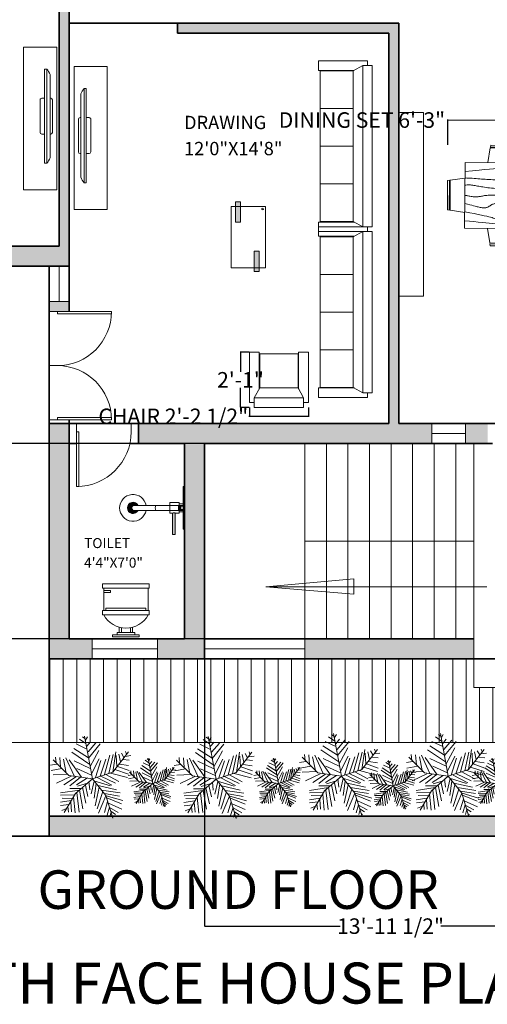
# Model space of a CAD drawing. Units: inches. Extents: x 1319 to 2030, y 219 to 1069.
# Tile 21 of 28: x 1565 to 1776, y 219 to 663. Entities that reach past the tile are written whole.
import ezdxf

# ---------------------------------------------------------------- set-up
doc = ezdxf.new("R2010")
doc.units = ezdxf.units.IN
doc.header["$MEASUREMENT"] = 0
doc.layers.get('0').update_dxf_attribs({"color": 12})
for name, color, linetype, lineweight in [('A-ANNO-DIMS', 2, 'Continuous', 18), ('A-AREA-IDEN', 250, 'Continuous', 18), ('A-FLOR', 8, 'Continuous', 18), ('A-FLOR-CASE', 8, 'Continuous', 18), ('A-FLOR-PATT', 41, 'Continuous', 13), ('A-FLOR-STRS', 7, 'Continuous', 18), ('A-GLAZ', 4, 'Continuous', 18), ('A-WALL-PATT', 252, 'Continuous', 13), ('C-PROP', 7, 'Continuous', 35), ('doors', 252, 'Continuous', 18), ('furniture', 250, 'Continuous', 18), ('lawn', 82, 'Continuous', 13), ('PLUMBING FIXTURES', 252, 'Continuous', 18), ('text', 7, 'Continuous', 25), ('walls', 250, 'Continuous', 35)]:
    doc.layers.add(name, color=color, linetype=linetype, lineweight=lineweight)
doc.styles.get("Standard").update_dxf_attribs({"font": 'arial.ttf'})
doc.dimstyles.get("Standard").update_dxf_attribs({"dimtxt": 7, "dimasz": 0.18, "dimexe": 0.18, "dimexo": 0.0625, "dimgap": 0.09, "dimtad": 0, "dimtih": 1, "dimtoh": 1, "dimzin": 0, "dimdsep": 46, "dimlunit": 3, "dimtxsty": 'Standard', "dimcen": 0.09, "dimadec": 0, "dimazin": 0, "dimtfac": 1, "dimtofl": 0, "dimtmove": 0, "dimatfit": 3, "dimfxl": 1, "dimtolj": 1, "dimtzin": 0, "dimarcsym": 0})

# ---------------------------------------------------------------- blocks, each defined once
blk = doc.blocks.new('*U2')
for p, q in [((0, 0), (0, -6)), ((40, 0), (40, -6))]:
    blk.add_line(p, q)
blk.add_lwpolyline([(0, 0), (0, 40), (1.75, 40), (1.75, 0)], close=True)
blk.add_arc((0, 0), 40, 0, 90)
blk = doc.blocks.new('Dining Set - 36 x 72 in.')
for p, q in [((-22, 27.5), (-22.1562, 26.50042)), ((-22, 27.5), (-6, 27.5)), ((-5.8437, 26.49966), (-6, 27.5)), ((6, 27.5), (5.8438, 26.50042)), ((6, 27.5), (22, 27.5)), ((22.1563, 26.49966), (22, 27.5)), ((-22.2343, 26.00059), (-23.4847, 17.99762)), ((-22.2304, 26), (-5.7608, 26)), ((-5.8416, 26.5), (-22.1534, 26.5)), ((-4.5152, 17.99762), (-5.7655, 25.99926)), ((5.7657, 26.00059), (4.5153, 17.99762)), ((5.7696, 26), (22.2392, 26)), ((22.1584, 26.5), (5.8466, 26.5)), ((23.4848, 17.99762), (22.2345, 25.99926)), ((36, 18), (-36, 18)), ((-36, 18), (-36, -18)), ((36, -18), (36, 18)), ((-45.5, 8), (-44.5004, 8.15617)), ((-45.5, 8), (-45.5, -8)), ((-44.5, -8.15843), (-44.5, 8.15338)), ((-44.0006, 8.23428), (-35.9976, 9.48474)), ((-44, 8.23041), (-44, -8.23915)), ((44.0006, 8.23428), (35.9976, 9.48474)), ((44, 8.23041), (44, -8.23915)), ((44.5, -8.15843), (44.5, 8.15338)), ((45.5, 8), (44.5005, 8.15617)), ((45.5, 8), (45.5, -8)), ((-44.4997, -8.15631), (-45.5, -8)), ((-35.9976, -9.48476), (-43.9993, -8.2345)), ((35.9976, -9.48476), (43.9993, -8.2345)), ((44.4997, -8.15631), (45.5, -8)), ((-36, -18), (36, -18)), ((-22.2343, -26.0006), (-23.4847, -17.99762)), ((-4.5152, -17.99762), (-5.7655, -25.99928)), ((5.7657, -26.0006), (4.5153, -17.99762)), ((23.4848, -17.99762), (22.2345, -25.99928)), ((-22.2304, -26), (-5.7608, -26)), ((-22, -27.5), (-22.1562, -26.50044)), ((-5.8416, -26.5), (-22.1534, -26.5)), ((-5.8437, -26.49967), (-6, -27.5)), ((5.7696, -26), (22.2392, -26)), ((6, -27.5), (5.8438, -26.50044)), ((22.1584, -26.5), (5.8466, -26.5)), ((22.1563, -26.49967), (22, -27.5)), ((-22, -27.5), (-6, -27.5)), ((6, -27.5), (22, -27.5))]:
    blk.add_line(p, q)
for points in [[(-36, 15), (-31.1772, 14.97754), (-26.8079, 14.91406), (-22.8538, 14.81543), (-19.276, 14.6875), (-16.0362, 14.53613), (-13.0957, 14.36718), (-10.4159, 14.18652), (-7.9583, 14), (-5.6904, 13.81315), (-3.6035, 13.63021), (-1.6954, 13.45508), (0.0365, 13.29166), (1.5945, 13.14388), (2.9811, 13.01562), (4.1988, 12.9108), (5.25, 12.83333), (6.1393, 12.78613), (6.8802, 12.76823), (7.4883, 12.77767), (7.9792, 12.8125), (8.3685, 12.87077), (8.6719, 12.95052), (8.9049, 13.0498), (9.0833, 13.16666), (9.2205, 13.29899), (9.3216, 13.44401), (9.3895, 13.59879), (9.4271, 13.76041), (9.4373, 13.92594), (9.4232, 14.09245), (9.3875, 14.257), (9.3333, 14.41666), (9.2638, 14.56917), (9.1836, 14.71484), (9.0975, 14.85465), (9.0104, 14.98958), (8.9272, 15.1206), (8.8529, 15.2487), (8.7922, 15.37483), (8.75, 15.5), (8.7305, 15.62467), (8.7344, 15.74739), (8.7617, 15.86621), (8.8125, 15.97916), (8.8867, 16.08431), (8.9844, 16.17968), (9.1055, 16.26334), (9.25, 16.33333), (9.4189, 16.38802), (9.6172, 16.42708), (9.8506, 16.45052), (10.125, 16.45833), (10.4463, 16.45052), (10.8203, 16.42708), (11.2529, 16.38802), (11.75, 16.33333), (12.3184, 16.26318), (12.9694, 16.17838), (13.7151, 16.07991), (14.5677, 15.96875), (15.5395, 15.84586), (16.6426, 15.71224), (17.8893, 15.56884), (19.2917, 15.41666), (20.859, 15.25667), (22.5879, 15.08984), (24.4721, 14.91715), (26.5052, 14.73958), (28.6809, 14.5581), (30.9929, 14.3737), (33.4347, 14.18733), (36, 14)], [(-36, 10), (-28.9766, 10.14274), (-23.1725, 10.20442), (-18.4241, 10.19775), (-14.5677, 10.13541), (-11.4399, 10.03011), (-8.877, 9.89453), (-6.7154, 9.74137), (-4.7917, 9.58333), (-2.9698, 9.43082), (-1.2246, 9.28515), (0.4415, 9.14534), (2.026, 9.01041), (3.5266, 8.87939), (4.9408, 8.7513), (6.266, 8.62516), (7.5, 8.5), (8.6411, 8.37549), (9.6914, 8.2539), (10.6538, 8.13818), (11.5312, 8.03125), (12.3267, 7.93603), (13.043, 7.85547), (13.6831, 7.79248), (14.25, 7.75), (14.7471, 7.7303), (15.1797, 7.73307), (15.5537, 7.75732), (15.875, 7.80208), (16.1494, 7.86637), (16.3828, 7.94922), (16.5811, 8.04964), (16.75, 8.16666), (16.8944, 8.29915), (17.0143, 8.44531), (17.1089, 8.60319), (17.1771, 8.77083), (17.218, 8.94629), (17.2305, 9.1276), (17.2137, 9.31282), (17.1667, 9.5), (17.0895, 9.6875), (16.987, 9.875), (16.8649, 10.0625), (16.7292, 10.25), (16.5856, 10.4375), (16.4401, 10.625), (16.2985, 10.8125), (16.1667, 11), (16.05, 11.18733), (15.9518, 11.3737), (15.8752, 11.5581), (15.8229, 11.73958), (15.798, 11.91715), (15.8034, 12.08984), (15.842, 12.25667), (15.9167, 12.41666), (16.0295, 12.56836), (16.1784, 12.70833), (16.3605, 12.83268), (16.5729, 12.9375), (16.8127, 13.01888), (17.0768, 13.07291), (17.3625, 13.0957), (17.6667, 13.08333), (17.9894, 13.03312), (18.3418, 12.94726), (18.7382, 12.82918), (19.1927, 12.68229), (19.7195, 12.51001), (20.3327, 12.31575), (21.0465, 12.10294), (21.875, 11.875), (22.8357, 11.63354), (23.959, 11.37304), (25.2786, 11.08618), (26.8282, 10.76562), (28.6414, 10.40405), (30.752, 9.99414), (33.1936, 9.52856), (36, 9)], [(-36, 5.5), (-30.7157, 5.3348), (-26.069, 5.20963), (-21.9946, 5.11767), (-18.4271, 5.05208), (-15.3009, 5.00602), (-12.5508, 4.97265), (-10.1112, 4.94515), (-7.9167, 4.91666), (-5.909, 4.88167), (-4.0586, 4.83984), (-2.3429, 4.79215), (-0.7396, 4.73958), (0.7739, 4.6831), (2.22, 4.6237), (3.6213, 4.56233), (5, 4.5), (6.373, 4.43782), (7.7344, 4.3776), (9.0723, 4.32129), (10.375, 4.27083), (11.6309, 4.22819), (12.8281, 4.19531), (13.9551, 4.17415), (15, 4.16666), (15.954, 4.17448), (16.819, 4.19791), (17.6001, 4.23698), (18.3021, 4.29166), (18.9299, 4.36198), (19.4883, 4.44791), (19.9823, 4.54948), (20.4167, 4.66666), (20.7969, 4.79899), (21.1302, 4.94401), (21.4245, 5.09879), (21.6875, 5.26041), (21.9271, 5.42594), (22.1511, 5.59245), (22.3672, 5.757), (22.5834, 5.91666), (22.8065, 6.06868), (23.0404, 6.21093), (23.2879, 6.34147), (23.5521, 6.45833), (23.8358, 6.55957), (24.142, 6.64323), (24.4735, 6.70735), (24.8334, 6.75), (25.2235, 6.76969), (25.642, 6.76692), (26.0858, 6.74267), (26.5521, 6.69791), (27.0379, 6.63362), (27.5404, 6.55078), (28.0565, 6.45036), (28.5834, 6.33333), (29.1242, 6.19987), (29.7071, 6.04687), (30.3661, 5.87044), (31.1354, 5.66666), (32.0493, 5.43164), (33.142, 5.16146), (34.4475, 4.85221), (36, 4.5)], [(-36, -1), (-30.7915, -0.6591), (-26.0195, -0.38216), (-21.6519, -0.16284), (-17.6563, 0.00521), (-14.0005, 0.12833), (-10.6523, 0.21289), (-7.5796, 0.26522), (-4.75, 0.29166), (-2.134, 0.29793), (0.2878, 0.28711), (2.5317, 0.26163), (4.6146, 0.22396), (6.5529, 0.17651), (8.3633, 0.12174), (10.0623, 0.06209), (11.6667, 0), (13.1899, -0.06201), (14.6341, -0.1211), (15.9982, -0.17432), (17.2813, -0.21875), (18.4823, -0.25147), (19.6003, -0.26953), (20.6343, -0.27002), (21.5834, -0.25), (22.4481, -0.20768), (23.2357, -0.14584), (23.9549, -0.06836), (24.6146, 0.02083), (25.2235, 0.11784), (25.7904, 0.21875), (26.3241, 0.31966), (26.8334, 0.41666), (27.3265, 0.50618), (27.8099, 0.58593), (28.2894, 0.65397), (28.7709, 0.70833), (29.2601, 0.74707), (29.763, 0.76823), (30.2855, 0.76985), (30.8334, 0.75), (31.4088, 0.70784), (31.9994, 0.64713), (32.589, 0.57275), (33.1615, 0.48958), (33.7008, 0.4025), (34.1908, 0.3164), (34.6153, 0.23616), (34.9584, 0.16666), (35.2099, 0.11165), (35.3848, 0.07031), (35.504, 0.04069), (35.5886, 0.02083), (35.6594, 0.00879), (35.7377, 0.0026), (35.8442, 0.00032), (36, 0)], [(-36, -6.5), (-27.1843, -6.31267), (-20.084, -6.1263), (-14.469, -5.9419), (-10.1094, -5.76042), (-6.7752, -5.58285), (-4.2363, -5.41016), (-2.2629, -5.24333), (-0.625, -5.08334), (0.8708, -4.93099), (2.2715, -4.78646), (3.5872, -4.64974), (4.8281, -4.52084), (6.0046, -4.39974), (7.127, -4.28646), (8.2053, -4.18099), (9.25, -4.08334), (10.2705, -3.99382), (11.2734, -3.91407), (12.2647, -3.84603), (13.25, -3.79167), (14.2354, -3.75293), (15.2266, -3.73177), (16.2295, -3.73015), (17.25, -3.75), (18.2912, -3.79248), (19.3451, -3.85547), (20.4009, -3.93604), (21.4479, -4.03125), (22.4754, -4.13819), (23.4727, -4.25391), (24.4289, -4.37549), (25.3334, -4.5), (26.1785, -4.62492), (26.9694, -4.74935), (27.7145, -4.87281), (28.4219, -4.99479), (29.1, -5.11483), (29.7572, -5.23242), (30.4016, -5.34709), (31.0417, -5.45834), (31.6837, -5.56437), (32.3262, -5.65821), (32.9658, -5.73153), (33.599, -5.77604), (34.2224, -5.78345), (34.8327, -5.74545), (35.4264, -5.65373), (36, -5.5)], [(-36, -10), (-26.4022, -9.81299), (-18.4675, -9.62891), (-11.9839, -9.45069), (-6.7396, -9.28125), (-2.5226, -9.12354), (0.8789, -8.98047), (3.6769, -8.85498), (6.0833, -8.75), (8.2767, -8.66765), (10.3021, -8.60677), (12.1712, -8.56543), (13.8958, -8.54167), (15.4876, -8.53353), (16.9583, -8.53907), (18.3197, -8.55632), (19.5834, -8.58334), (20.7616, -8.61841), (21.8685, -8.66081), (22.9188, -8.71004), (23.9271, -8.76563), (24.9081, -8.82707), (25.8763, -8.89388), (26.8465, -8.96558), (27.8334, -9.04167), (28.8474, -9.12118), (29.8828, -9.20117), (30.93, -9.27824), (31.9792, -9.34896), (33.0205, -9.40991), (34.0443, -9.45768), (35.0407, -9.48885), (36, -9.5)], [(-36, -14.5), (-30.0881, -14.33513), (-25.0332, -14.21224), (-20.7312, -14.12647), (-17.0781, -14.07292), (-13.97, -14.04671), (-11.3027, -14.04297), (-8.9724, -14.05681), (-6.875, -14.08334), (-4.9224, -14.11833), (-3.0905, -14.16016), (-1.3709, -14.20785), (0.2448, -14.26042), (1.7647, -14.3169), (3.1973, -14.3763), (4.5507, -14.43767), (5.8333, -14.5), (7.0554, -14.5621), (8.235, -14.62175), (9.3922, -14.67652), (10.5469, -14.72396), (11.7192, -14.76164), (12.929, -14.78711), (14.1965, -14.79794), (15.5417, -14.79167), (16.9933, -14.76424), (18.6152, -14.70508), (20.4804, -14.60197), (22.6615, -14.44271), (25.2312, -14.21509), (28.2624, -13.9069), (31.8277, -13.50594), (36, -13)]]:
    blk.add_lwpolyline(points)
blk = doc.blocks.new('dining area')
at = {"layer": 'furniture', "xscale": 0.6659924291999282, "yscale": 0.6659924291999282, "zscale": 0.6659924291999282, "rotation": 90}
blk.add_blockref('Dining Set - 36 x 72 in.', (-0.44, 20.51), dxfattribs=at)
blk = doc.blocks.new('FABRIC SOFA 1S')
at = {"layer": 'furniture'}
for p, q in [((0, -15.12), (0, 15.12)), ((6, 15.12), (0, 15.12)), ((3, 18.12), (34, 18.12)), ((3, 15.12), (3, 18.12)), ((6, -15.12), (6, 15.12)), ((12, 11.75), (6, 15.12)), ((11.33, 12.12), (34, 12.12)), ((34, 12.12), (34, 18.12)), ((6, -15.12), (12, -11.75)), ((6, -15.12), (0, -15.12)), ((3, -18.12), (3, -15.12)), ((3, -18.12), (34, -18.12)), ((11.33, -12.12), (34, -12.12)), ((34, -12.12), (34, -18.12))]:
    blk.add_line(p, q, dxfattribs=at)
blk.add_lwpolyline([(12, -11.75), (12, 11.75), (33, 11.75), (33, -11.75)], close=True, dxfattribs=at)
blk = doc.blocks.new('FABRIC SOFA 4S')
at = {"layer": 'furniture'}
for p, q in [((0, -51), (0, 51)), ((6, 51), (0, 51)), ((3, 54), (34, 54)), ((3, 51), (3, 54)), ((6, -51), (6, 51)), ((12, 47.63), (6, 51)), ((34, 48), (34, 54)), ((11.14, 48), (34, 48)), ((33, 23.81), (12, 23.81)), ((33, 0), (12, 0)), ((33, -23.81), (12, -23.81)), ((6, -51), (12, -47.63)), ((11.54, -48), (34, -48)), ((34, -48), (34, -54)), ((6, -51), (0, -51)), ((3, -54), (3, -51)), ((3, -54), (34, -54))]:
    blk.add_line(p, q, dxfattribs=at)
blk.add_lwpolyline([(12, -47.63), (12, 47.63), (33, 47.63), (33, -47.63)], close=True, dxfattribs=at)
blk = doc.blocks.new('O.H SHOWER-PL')
at = {"layer": 'PLUMBING FIXTURES'}
for points in [[(-1.84, 0), (-1.84, -0.25), (1.84, -0.25), (1.84, 0)], [(0.46, -8.72), (0.46, -9.67, -0.422337), (-0.46, -9.67), (-0.46, -8.72, 4.325472)]]:
    blk.add_hatch(color=256, dxfattribs=at).paths.add_polyline_path(points)
for p, q in [((-1.84, 0), (-1.84, -0.25)), ((1.84, 0), (-1.84, 0)), ((1.84, 0), (1.84, -0.25)), ((1.84, -0.25), (-1.84, -0.25)), ((-0.46, -0.25), (-0.46, -9.67)), ((0.46, -0.25), (0.46, -9.67))]:
    blk.add_line(p, q, dxfattribs=at)
for centre, radius, start, end in [((0, -4.48), 1.03, 243.53, 296.47), ((0, -9.67), 2.5, 100.61, 79.39), ((0, -9.67), 1.05, 116.0349, 63.9652), ((0, -9.22), 0.643, 224.2078, 315.7922)]:
    blk.add_arc(centre, radius, start, end, dxfattribs=at)
blk = doc.blocks.new('DIVERTER-PL')
at = {"layer": 'PLUMBING FIXTURES'}
for points in [[(4, 0), (-4, 0), (-4, -0.25), (4, -0.25)], [(0.38, -1.14), (0.38, -0.7), (-0.37, -0.7), (-0.37, -1.14)], [(1, -1.75, 0.30818), (1, -2.25), (5, -2.25), (5, -1.75)]]:
    blk.add_hatch(color=256, dxfattribs=at).paths.add_polyline_path(points)
for p, q in [((-4, 0), (-4, -0.25)), ((-4, 0), (4, 0)), ((4, 0), (4, -0.25)), ((-4, -0.25), (4, -0.25)), ((-4, -0.25), (4, -0.25)), ((-1, -1.05), (-0.37, -1.05)), ((-1, -1.05), (-1, -2.75)), ((-0.75, -0.25), (-0.75, -1.05)), ((-0.37, -0.7), (0.38, -0.7)), ((-0.37, -0.7), (-0.37, -1.14)), ((-0.37, -1.14), (0.38, -1.14)), ((-0.32, -0.7), (-0.32, -0.25)), ((0.32, -0.7), (0.32, -0.25)), ((0.38, -0.7), (0.38, -1.14)), ((0.38, -1.05), (1, -1.05)), ((0.75, -0.25), (0.75, -1.05)), ((1, -1.05), (1, -1.75)), ((-1, -2.75), (1, -2.75)), ((1, -2.25), (1, -2.75))]:
    blk.add_line(p, q, dxfattribs=at)
at = {"layer": 'PLUMBING FIXTURES', "ltscale": 12}
for p, q in [((1, -1.75), (5, -1.75)), ((5, -2.25), (5, -1.75)), ((1, -2.25), (5, -2.25))]:
    blk.add_line(p, q, dxfattribs=at)
at = {"layer": 'PLUMBING FIXTURES'}
blk.add_arc((1.37, -2), 0.444, 145.7435, 214.2565, dxfattribs=at)
blk = doc.blocks.new('A$C7F153053')
at = {"layer": 'PLUMBING FIXTURES', "xscale": -1, "rotation": 270}
for name in ['DIVERTER-PL', 'O.H SHOWER-PL']:
    blk.add_blockref(name, (12.17, 4), dxfattribs=at)
blk = doc.blocks.new('*U25')
for p, q in [((-10, 22), (-10, 12)), ((-10, 21), (-7, 21)), ((-7, 20), (-10, 20)), ((-7, 21), (-7, 20)), ((10, 12), (10, 22)), ((10.5, 12), (-10.5, 12)), ((-10.5, 10), (-10.5, 12)), ((10.5, 10), (-10.5, 10)), ((9, 13), (-9, 13)), ((-9, 13), (-9, 12)), ((9, 12), (9, 13)), ((10.5, 12), (10.5, 10)), ((4, 2), (-4, 2)), ((-4, 2), (-4, 1)), ((-3, 4.4065), (-3, 2)), ((-2, 2), (-2, 4.1658)), ((2, 4.1658), (2, 2)), ((3, 2), (3, 4.4065)), ((4, 1), (4, 2))]:
    blk.add_line(p, q)
for points in [[(10.5, 22), (10.5, 24), (-10.5, 24), (-10.5, 22)], [(6, 0), (6, 1), (-6, 1), (-6, 0)]]:
    blk.add_lwpolyline(points, close=True)
blk.add_arc((0, 15.3333), 11.3333, 208.0725, 331.9275)
blk = doc.blocks.new('*U27')
for p, q in [((-8.737, 47.138), (-17.069, 52.711)), ((-10.186, 53.64), (-13.084, 55.962)), ((0, 0), (-10.5, 57)), ((-9.099, 51.782), (-6.563, 55.962)), ((-5.114, 28.097), (-24.676, 40.636)), ((-7.288, 39.707), (-21.778, 46.673)), ((-7.65, 43.423), (-2.578, 49.46)), ((-5.839, 35.992), (4.667, 48.067)), ((-5.114, 27.632), (10.463, 46.673)), ((-48.585, 21.131), (-49.309, 29.026)), ((-43.513, 28.561), (-42.427, 15.558)), ((-35.544, 28.097), (-24.314, 3.947)), ((-3.665, 19.273), (-27.574, 35.527)), ((-2.941, 16.486), (8.652, 37.85)), ((-1.129, 6.734), (9.014, 26.704)), ((16.259, 5.805), (23.142, 31.348)), ((22.055, 7.198), (27.489, 32.277)), ((27, 9), (48, 36)), ((27.127, 9.056), (31.112, 35.992)), ((31.836, 30.883), (32.561, 16.486)), ((35.096, 32.741), (37.27, 22.524)), ((38.719, 34.134), (41.979, 28.561)), ((43.791, 29.954), (51.036, 30.883)), ((44.153, 36.456), (45.239, 32.741)), ((-47.498, 19.737), (-55.83, 18.344)), ((-40.615, 13.7), (-55.105, 10.913)), ((-31.5, 4.5), (-52.5, 25.5)), ((-38.442, 26.239), (-34.819, 7.663)), ((-14.533, 2.09), (-30.834, 25.31)), ((-24.314, 23.917), (-2.941, 13.7)), ((-20.691, 13.7), (-1.129, 4.876)), ((3.942, 1.625), (11.187, 24.381)), ((10.101, 3.483), (17.708, 26.239)), ((33.285, 16.486), (48.862, 10.913)), ((36.183, 19.737), (48.137, 17.88)), ((40.53, 25.775), (48.862, 24.846)), ((-33.37, 6.269), (-52.207, 5.34)), ((-28.299, 3.483), (-47.86, -5.805)), ((-21.416, 3.018), (-38.079, -8.128)), ((0, 0), (-31.5, 4.5)), ((-15.982, 2.09), (-30.11, -9.521)), ((0, 0), (-22.5, -19.5)), ((-6.563, 1.161), (-21.416, -8.128)), ((0, 0), (27, 9)), ((0, 0), (18, -22.5)), ((6.478, 1.625), (26.04, -8.592)), ((11.187, 3.483), (30.749, -5.805)), ((18.07, 5.805), (35.096, -3.483)), ((24.229, 7.663), (46.688, 1.625)), ((29.662, 12.307), (48.137, 6.269)), ((-15.257, -12.772), (-30.11, -12.772)), ((-6.563, -5.805), (-19.967, -9.985)), ((-13.446, -11.378), (-8.737, -32.741)), ((-9.461, -8.592), (-6.201, -23.453)), ((-4.752, -3.483), (-3.665, -14.629)), ((2.493, -3.019), (-1.491, -20.202)), ((1.769, -2.555), (24.229, -9.521)), ((5.029, -6.27), (2.131, -25.775)), ((9.014, -11.378), (3.58, -35.992)), ((7.565, -9.056), (32.198, -14.629)), ((-17.431, -15.094), (-42.789, -18.809)), ((-24.314, -21.596), (-42.427, -22.06)), ((-26.849, -26.24), (-40.253, -25.775)), ((-22.5, -19.5), (-37.5, -45)), ((-25.038, -23.918), (-22.865, -45.281)), ((-20.691, -18.345), (-17.793, -44.352)), ((-17.069, -15.094), (-12.721, -40.172)), ((14.085, -16.951), (6.478, -40.172)), ((18.07, -22.524), (8.289, -45.745)), ((12.274, -15.094), (36.907, -18.809)), ((16.259, -19.738), (36.183, -22.989)), ((18, -22.5), (27, -52.5)), ((18.433, -22.524), (40.53, -29.026)), ((19.157, -25.311), (38.719, -33.206)), ((-28.299, -29.026), (-42.789, -31.348)), ((-30.834, -34.135), (-42.427, -35.528)), ((-32.646, -36.921), (-31.921, -44.352)), ((-29.023, -30.884), (-27.936, -43.887)), ((20.244, -30.419), (15.897, -44.816)), ((22.78, -37.85), (19.519, -48.532)), ((21.331, -32.741), (39.081, -40.636)), ((22.78, -38.314), (34.372, -44.816)), ((-34.457, -39.708), (-40.978, -42.494)), ((24.591, -45.745), (23.142, -50.854)), ((24.591, -43.423), (30.749, -47.603)), ((26.764, -49.925), (28.213, -50.854))]:
    blk.add_line(p, q)
blk = doc.blocks.new('TABLE-COCKTAIL')
h = blk.add_hatch(color=256)
h.dxf.hatch_style = 1
h.paths.add_polyline_path([(4.23, 29.31), (2.04, 29.31), (2.04, 22.19), (4.23, 22.19)])
h.paths.add_polyline_path([(4.23, 31.28), (2.04, 31.28), (2.04, 29.31), (4.23, 29.31)])
h.paths.add_polyline_path([(12.58, 9.09), (10.39, 9.09), (10.39, 1.62), (12.58, 1.62)])
h.paths.add_polyline_path([(12.58, 1.62), (10.39, 1.62), (10.39, 0), (12.58, 0)])
for p, q in [((2.04, 31.28), (4.23, 31.28)), ((2.04, 22.19), (2.04, 31.28)), ((4.23, 31.28), (4.23, 22.19)), ((0, 29.31), (0, 1.62)), ((15.53, 29.31), (0, 29.31)), ((15.53, 1.62), (15.53, 29.31)), ((4.23, 22.19), (2.04, 22.19)), ((10.39, 9.09), (12.58, 9.09)), ((10.39, 0), (10.39, 9.09)), ((12.58, 9.09), (12.58, 0)), ((0, 1.62), (15.53, 1.62)), ((12.58, 0), (10.39, 0))]:
    blk.add_line(p, q)
blk.add_circle((14.17, 28.1), 0.401)
blk = doc.blocks.new('PLASMA-LARGE')
at = {"layer": 'furniture'}
for p, q in [((-7.26, 0), (7.26, 0)), ((-21, -2.5), (21, -2.5)), ((-21, -2.5), (-21, -3.5)), ((-21, -3.5), (21, -3.5)), ((-18.61, -1), (18.61, -1)), ((-8, -1), (-8, -0.74)), ((-8, -3.5), (-8, -4.76)), ((8, -1), (8, -0.74)), ((8, -3.5), (8, -4.76)), ((21, -2.5), (21, -3.5)), ((-7.26, -5.5), (7.26, -5.5))]:
    blk.add_line(p, q, dxfattribs=at)
for centre, radius, start, end in [((-7.26, -0.74), 0.744, 90, 180), ((7.26, -0.74), 0.744, 0, 90), ((-13.97, -11.05), 11.07, 114.7602, 129.4175), ((13.97, -11.05), 11.07, 50.5825, 65.2398), ((-7.26, -4.76), 0.744, 180, 270), ((7.26, -4.76), 0.744, 270, 0)]:
    blk.add_arc(centre, radius, start, end, dxfattribs=at)
blk = doc.blocks.new('MEDIA-CONSOLE')
for p, q in [((64.44, 14.9), (0, 14.9)), ((0, 14.9), (0, 0)), ((64.44, 0), (64.44, 14.9)), ((0, 0), (64.44, 0))]:
    blk.add_line(p, q)
at = {"xscale": -1.011294184530666, "yscale": 1.011294184530666, "zscale": 1.011294184530666, "rotation": 180}
blk.add_blockref('PLASMA-LARGE', (33.26, 1.95), dxfattribs=at)
blk = doc.blocks.new('*D54')
at = {"layer": 'A-ANNO-DIMS', "color": 0, "lineweight": -2, "transparency": 16777216}
for p, q in [((1757.94, 618.08), (1757.76, 618.08)), ((1757.87, 606.9), (1757.94, 618.26)), ((1832.71, 617.63), (1758.12, 618.08)), ((1832.82, 606.45), (1832.89, 617.81))]:
    blk.add_line(p, q, dxfattribs=at)
at = {"layer": 'A-ANNO-DIMS', "color": 0, "transparency": 16777216}
for points in [[(1758.12, 618.11), (1758.12, 618.05), (1757.94, 618.08)], [(1832.71, 617.66), (1832.71, 617.6), (1832.89, 617.63)]]:
    blk.add_solid(points, dxfattribs=at)
at = {"layer": 'Defpoints', "color": 0, "transparency": 16777216}
for p in [(1757.94, 618.08), (1757.87, 606.84), (1832.82, 606.38)]:
    blk.add_point(p, dxfattribs=at)
at = {"layer": 'A-ANNO-DIMS', "color": 0, "transparency": 16777216, "insert": (1719.2, 618.08), "char_height": 7, "attachment_point": 5}
blk.add_mtext('\\A1;DINING SET 6\'-3"', dxfattribs=at)
blk = doc.blocks.new('*D60')
at = {"layer": 'A-ANNO-DIMS', "color": 0, "lineweight": -2, "transparency": 16777216}
for p, q in [((1668.5, 488.43), (1668.5, 484.32)), ((1695.11, 488.43), (1695.11, 484.32)), ((1668.5, 484.5), (1668.32, 484.5)), ((1694.93, 484.5), (1668.68, 484.5))]:
    blk.add_line(p, q, dxfattribs=at)
at = {"layer": 'A-ANNO-DIMS', "color": 0, "transparency": 16777216}
for points in [[(1668.68, 484.53), (1668.68, 484.47), (1668.5, 484.5)], [(1694.93, 484.53), (1694.93, 484.47), (1695.11, 484.5)]]:
    blk.add_solid(points, dxfattribs=at)
at = {"layer": 'Defpoints', "color": 0, "transparency": 16777216}
for p in [(1668.5, 488.49), (1695.11, 488.49), (1668.5, 484.5)]:
    blk.add_point(p, dxfattribs=at)
at = {"layer": 'A-ANNO-DIMS', "color": 0, "transparency": 16777216, "insert": (1634.24, 484.5), "char_height": 7, "attachment_point": 5}
blk.add_mtext('\\A1;CHAIR 2\'-2 1/2"', dxfattribs=at)
blk = doc.blocks.new('*D61')
at = {"layer": 'A-ANNO-DIMS', "color": 0, "lineweight": -2, "transparency": 16777216}
for p, q in [((1668.44, 513.45), (1664.33, 513.45)), ((1664.51, 513.27), (1664.51, 504.58)), ((1664.51, 488.67), (1664.51, 497.37)), ((1668.44, 488.49), (1664.33, 488.49))]:
    blk.add_line(p, q, dxfattribs=at)
at = {"layer": 'A-ANNO-DIMS', "color": 0, "transparency": 16777216}
for points in [[(1664.48, 513.27), (1664.54, 513.27), (1664.51, 513.45)], [(1664.48, 488.67), (1664.54, 488.67), (1664.51, 488.49)]]:
    blk.add_solid(points, dxfattribs=at)
at = {"layer": 'Defpoints', "color": 0, "transparency": 16777216}
for p in [(1664.51, 513.45), (1668.5, 513.45), (1668.5, 488.49)]:
    blk.add_point(p, dxfattribs=at)
at = {"layer": 'A-ANNO-DIMS', "color": 0, "transparency": 16777216, "insert": (1664.51, 500.97), "char_height": 7, "attachment_point": 5}
blk.add_mtext('\\A1;2\'-1"', dxfattribs=at)
blk = doc.blocks.new('*D64')
at = {"layer": 'A-ANNO-DIMS', "color": 0, "lineweight": -2, "transparency": 16777216}
for p, q in [((1648.34, 375.16), (1648.34, 254.5)), ((1815.84, 375.16), (1815.84, 254.5)), ((1648.52, 254.68), (1709.43, 254.68)), ((1815.66, 254.68), (1754.75, 254.68))]:
    blk.add_line(p, q, dxfattribs=at)
at = {"layer": 'A-ANNO-DIMS', "color": 0, "transparency": 16777216}
for points in [[(1648.52, 254.71), (1648.52, 254.65), (1648.34, 254.68)], [(1815.66, 254.71), (1815.66, 254.65), (1815.84, 254.68)]]:
    blk.add_solid(points, dxfattribs=at)
at = {"layer": 'Defpoints', "color": 0, "transparency": 16777216}
for p in [(1648.34, 375.23), (1815.84, 375.23), (1815.84, 254.68)]:
    blk.add_point(p, dxfattribs=at)
at = {"layer": 'A-ANNO-DIMS', "color": 0, "transparency": 16777216, "insert": (1732.09, 254.68), "char_height": 7, "attachment_point": 5}
blk.add_mtext('\\A1;13\'-11 1/2"', dxfattribs=at)
blk = doc.blocks.new('*D65')
at = {"layer": 'A-ANNO-DIMS', "color": 0, "lineweight": -2, "transparency": 16777216}
for p, q in [((1648.280254, 472.227245), (1329.112754, 472.227245)), ((1329.292754, 472.047245), (1329.292754, 431.817245)), ((1329.292754, 384.407245), (1329.292754, 424.637245)), ((1648.280254, 384.227245), (1329.112754, 384.227245))]:
    blk.add_line(p, q, dxfattribs=at)
at = {"layer": 'A-ANNO-DIMS', "color": 0, "transparency": 16777216}
for points in [[(1329.262754, 472.047245), (1329.322754, 472.047245), (1329.292754, 472.227245)], [(1329.262754, 384.407245), (1329.322754, 384.407245), (1329.292754, 384.227245)]]:
    blk.add_solid(points, dxfattribs=at)
at = {"layer": 'Defpoints', "color": 0, "transparency": 16777216}
for p in [(1329.292754, 472.227245), (1648.342754, 472.227245), (1648.342754, 384.227245)]:
    blk.add_point(p, dxfattribs=at)
at = {"layer": 'A-ANNO-DIMS', "color": 0, "transparency": 16777216, "insert": (1329.292754, 428.227245), "char_height": 7, "attachment_point": 5}
blk.add_mtext('\\A1;7\'-4"', dxfattribs=at)

msp = doc.modelspace()

# ---------------------------------------------------------------- hatches: boundary and pattern name
at = {"layer": 'A-FLOR-PATT'}
h = msp.add_hatch(dxfattribs=at)
h.set_pattern_fill('ANSI31', color=256, scale=48.3872, angle=45, style=0)
h.paths.add_polyline_path([(1578.343, 337.406), (1823.279, 337.406), (1823.279, 362.242), (1769.593, 362.242), (1769.593, 375.227), (1578.343, 375.227)])
at = {"layer": 'A-WALL-PATT'}
h = msp.add_hatch(color=256, dxfattribs=at)
h.dxf.hatch_style = 1
h.paths.add_polyline_path([(1378.843, 946.227), (1960.843, 946.227), (1960.843, 860.616), (1922.194, 860.616), (1922.194, 851.616), (1960.843, 851.616), (1960.843, 304.227), (1578.343, 304.227), (1578.343, 295.227), (1969.843, 295.227), (1969.843, 955.227), (1369.843, 955.227), (1369.843, 295.227), (1378.843, 295.227)])
h = msp.add_hatch(color=256, dxfattribs=at)
h.dxf.hatch_style = 1
h.paths.add_polyline_path([(1856.292, 860.616), (1812.343, 860.616), (1812.343, 851.616), (1812.343, 700.993), (1816.843, 700.993), (1816.843, 851.616), (1856.292, 851.616)])
h.paths.add_polyline_path([(1960.843, 663.616), (1812.343, 663.616), (1782.783, 663.616), (1782.783, 659.116), (1812.343, 659.116), (1960.843, 659.116)])
h.paths.add_polyline_path([(1857.424, 659.116), (1852.924, 659.116), (1852.924, 616.807), (1857.424, 616.807)])
h.paths.add_polyline_path([(1735.843, 661.727), (1731.843, 661.727), (1636.133, 661.727), (1636.133, 657.227), (1731.343, 657.227), (1731.343, 481.227), (1618.616, 481.227), (1618.616, 472.227), (1639.343, 472.227), (1639.343, 384.227), (1627.044, 384.227), (1627.044, 375.227), (1648.343, 375.227), (1648.343, 384.227), (1648.343, 472.227), (1750.706, 472.227), (1750.706, 481.227), (1735.843, 481.227), (1735.843, 657.727)])
h.paths.add_polyline_path([(1587.343, 481.227), (1578.343, 481.227), (1578.343, 375.227), (1597.622, 375.227), (1597.622, 384.227), (1587.343, 384.227)])
h.paths.add_polyline_path([(1769.593, 384.227), (1693.482, 384.227), (1693.482, 375.227), (1769.593, 375.227)])
h.paths.add_polyline_path([(1775.828, 481.227), (1765.831, 481.227), (1765.831, 472.227), (1775.828, 472.227)])
h.paths.add_polyline_path([(1824.625, 481.227), (1820.343, 481.227), (1820.343, 476.727), (1824.625, 476.727), (1824.625, 477.545)], flags=0)
h.paths.add_polyline_path([(1896.843, 481.227), (1852.26, 481.227), (1852.26, 476.727), (1892.343, 476.727), (1892.343, 384.227), (1881.742, 384.227), (1881.742, 375.227), (1913.435, 375.227), (1913.435, 384.227), (1896.843, 384.227)])
h.paths.add_polyline_path([(1960.843, 481.227), (1931.341, 481.227), (1931.341, 476.727), (1960.843, 476.727)])
h.paths.add_polyline_path([(1736.343, 918.227), (1731.843, 918.227), (1731.843, 890.227), (1582.843, 890.227), (1582.843, 781.727), (1582.843, 769.171), (1587.343, 769.171), (1587.343, 781.727), (1587.343, 885.727), (1731.843, 885.727), (1731.843, 851.616), (1736.343, 851.616), (1736.343, 890.227)])
h.paths.add_polyline_path([(1781.022, 860.616), (1773.021, 860.616, -0.0322281), (1773.289, 856.464), (1773.289, 851.616), (1781.022, 851.616)])
h.paths.add_polyline_path([(1587.343, 946.227), (1582.843, 946.227), (1582.843, 926.136), (1587.343, 926.136)])
h.paths.add_polyline_path([(1647.843, 946.227), (1643.343, 946.227), (1643.343, 926.136), (1647.843, 926.136)])
h.paths.add_polyline_path([(1543.343, 786.227), (1429.843, 786.227), (1429.843, 757.555), (1434.343, 757.555), (1438.843, 757.555), (1438.843, 781.727), (1543.343, 781.727)])
h.paths.add_polyline_path([(1543.343, 781.727), (1538.843, 781.727), (1538.843, 709.727), (1534.597, 709.727), (1534.597, 705.227), (1543.343, 705.227), (1543.343, 709.727)])
h.paths.add_polyline_path([(1499.955, 709.727), (1438.843, 709.727), (1438.843, 734.463), (1429.843, 734.463), (1429.843, 552.227), (1470.241, 552.227), (1470.241, 561.227), (1438.843, 561.227), (1438.843, 705.227), (1499.955, 705.227)])
h.paths.add_polyline_path([(1587.343, 709.727), (1582.843, 709.727), (1582.843, 561.227), (1543.433, 561.227), (1543.433, 552.227), (1587.343, 552.227)])
h.paths.add_polyline_path([(1546.835, 709.727), (1543.343, 709.727), (1543.343, 705.227), (1546.835, 705.227)])
h.paths.add_polyline_path([(1582.843, 709.727), (1579.15, 709.727), (1579.15, 705.227), (1582.843, 705.227)], flags=17)
h.paths.add_polyline_path([(1548.368, 786.227), (1543.343, 786.227), (1543.343, 781.727), (1548.368, 781.727)])
h.paths.add_polyline_path([(1582.843, 786.227), (1580.683, 786.227), (1580.683, 781.727), (1582.843, 781.727)])
h.paths.add_polyline_path([(1587.343, 892.402), (1582.843, 892.402), (1582.843, 890.227), (1587.343, 890.227)], flags=17)
h.paths.add_polyline_path([(1647.843, 892.402), (1643.343, 892.402), (1643.343, 890.227), (1647.843, 890.227)], flags=17)
h.paths.add_polyline_path([(1740.974, 856.464), (1740.974, 860.616), (1736.343, 860.616), (1736.343, 851.616), (1740.974, 851.616)])
h.paths.add_polyline_path([(1853.989, 384.227), (1820.343, 384.227), (1820.343, 402.924), (1815.843, 402.924), (1815.843, 375.227), (1853.989, 375.227)])
h.paths.add_polyline_path([(1892.343, 436.227), (1820.343, 436.227), (1820.343, 481.227), (1815.843, 481.227), (1815.843, 431.727), (1892.343, 431.727)])
h.paths.add_polyline_path([(1849.175, 481.227), (1824.625, 481.227), (1824.625, 477.545), (1825.699, 477.545), (1825.699, 453.018, 0.4014527), (1849.175, 477.545)], flags=0)
h.paths.add_polyline_path([(1960.843, 384.227), (1941.188, 384.227), (1941.188, 375.227), (1960.843, 375.227)])
h.paths.add_polyline_path([(1902.267, 481.227), (1896.843, 481.227), (1896.843, 476.727), (1902.267, 476.727), (1902.267, 477.44)], flags=0)
h = msp.add_hatch(color=256, dxfattribs=at)
h.dxf.hatch_style = 1
h.paths.add_polyline_path([(1587.343, 536.241), (1578.343, 536.241), (1578.343, 533.695), (1587.343, 533.695)])
h.paths.add_polyline_path([(1587.343, 533.695), (1578.343, 533.695), (1578.343, 531.767), (1582.004, 531.767), (1587.343, 531.767)])

# ---------------------------------------------------------------- linework, layer by layer
at = {"layer": 'A-FLOR'}
for p, q in [((1769.593, 362.242), (1823.279, 362.242)), ((1394.092, 337.406), (1817.431, 337.406))]:
    msp.add_line(p, q, dxfattribs=at)
at = {"layer": 'A-FLOR-CASE'}
for p, q in [((1735.843, 621.499), (1735.843, 621.499)), ((1735.843, 621.499), (1746.963, 621.499)), ((1746.963, 621.499), (1746.963, 538.752)), ((1746.963, 538.752), (1735.843, 538.752))]:
    msp.add_line(p, q, dxfattribs=at)
at = {"layer": 'A-FLOR-STRS'}
for p, q in [((1693.482, 384.227), (1693.482, 472.227)), ((1703.196, 384.227), (1703.196, 472.227)), ((1712.91, 384.227), (1712.91, 472.227)), ((1722.623, 384.227), (1722.623, 472.227)), ((1732.337, 384.227), (1732.337, 472.227)), ((1742.051, 384.227), (1742.051, 472.227)), ((1751.765, 384.227), (1751.765, 472.227)), ((1761.479, 384.227), (1761.479, 472.227)), ((1769.593, 472.227), (1769.593, 362.242)), ((1693.482, 428.227), (1769.593, 428.227)), ((1675.987, 407.684), (1715.617, 411.298)), ((1715.617, 411.298), (1715.617, 404.385)), ((1715.617, 404.385), (1675.987, 407.684)), ((1675.987, 407.684), (1715.617, 407.684)), ((1715.617, 407.684), (1775.534, 407.684))]:
    msp.add_line(p, q, dxfattribs=at)
at = {"layer": 'A-GLAZ'}
for p, q in [((1587.343, 552.227), (1578.343, 552.227)), ((1578.343, 552.227), (1578.343, 536.241)), ((1582.843, 536.241), (1582.843, 552.227)), ((1587.343, 536.241), (1587.343, 552.227)), ((1578.343, 536.241), (1587.343, 536.241)), ((1578.343, 536.241), (1582.843, 536.241)), ((1750.706, 481.227), (1750.706, 472.227)), ((1765.831, 481.227), (1750.706, 481.227)), ((1750.706, 481.227), (1750.706, 476.727)), ((1765.831, 472.227), (1765.831, 481.227)), ((1750.706, 476.727), (1765.831, 476.727)), ((1750.706, 472.227), (1765.831, 472.227)), ((1597.622, 384.227), (1597.622, 375.227)), ((1627.044, 384.227), (1597.622, 384.227)), ((1597.622, 384.227), (1597.622, 379.727)), ((1627.044, 375.227), (1627.044, 384.227)), ((1648.343, 384.227), (1693.482, 384.227)), ((1648.343, 375.227), (1648.343, 384.227)), ((1648.343, 384.227), (1648.343, 379.727)), ((1693.482, 384.227), (1693.482, 375.227)), ((1597.622, 379.727), (1627.044, 379.727)), ((1648.343, 379.727), (1693.482, 379.727)), ((1597.622, 375.227), (1627.044, 375.227)), ((1693.482, 375.227), (1648.343, 375.227))]:
    msp.add_line(p, q, dxfattribs=at)
at = {"layer": 'C-PROP'}
msp.add_line((1969.843, 295.227), (1369.843, 295.227), dxfattribs=at)
at = {"layer": 'walls'}
for p, q in [((1582.843, 561.227), (1582.843, 709.727)), ((1587.343, 531.767), (1587.343, 709.727)), ((1587.343, 661.727), (1731.843, 661.727)), ((1636.133, 661.727), (1636.133, 657.227)), ((1735.843, 661.727), (1731.843, 661.727)), ((1735.843, 657.727), (1735.843, 661.727)), ((1636.133, 657.227), (1731.343, 657.227)), ((1731.343, 481.227), (1731.343, 657.227)), ((1735.843, 481.227), (1735.843, 657.727)), ((1438.843, 561.227), (1582.843, 561.227)), ((1429.843, 552.227), (1587.343, 552.227)), ((1578.343, 295.227), (1578.343, 552.227)), ((1578.343, 481.227), (1731.343, 481.227)), ((1587.343, 481.227), (1587.343, 482.951)), ((1587.343, 384.227), (1587.343, 481.227)), ((1618.616, 481.227), (1618.616, 472.227)), ((1735.843, 481.227), (1960.843, 481.227)), ((1587.343, 472.227), (1590.592, 472.227)), ((1614.672, 472.227), (1639.343, 472.227)), ((1639.343, 384.227), (1639.343, 472.227)), ((1648.343, 375.227), (1648.343, 472.227)), ((1648.343, 472.227), (1777.989, 472.227)), ((1587.343, 384.227), (1639.343, 384.227)), ((1648.343, 384.227), (1769.593, 384.227)), ((1578.343, 375.227), (1960.843, 375.227)), ((1960.843, 304.227), (1578.343, 304.227))]:
    msp.add_line(p, q, dxfattribs=at)

# ---------------------------------------------------------------- block references
at = {"layer": 'doors'}
for p, xscale, yscale, zscale, rotation in [((1582.004, 531.767), 0.6102094931972349, 0.6102094931972349, 0.6102094931972349, 270), ((1582.004, 482.951), -0.6102094931972349, 0.6102094931972349, 0.6102094931972349, 270), ((1590.592, 477.529), -0.6164316052538731, 0.6164316052538731, 0.6164316052538731, 180)]:
    msp.add_blockref('*U2', p, dxfattribs=dict(at, xscale=xscale, yscale=yscale, zscale=zscale, rotation=rotation))
at = {"layer": 'furniture', "rotation": 89.99999999999969}
msp.add_blockref('MEDIA-CONSOLE', (1581.706, 586.572), dxfattribs=at)
at = {"layer": 'furniture'}
for name, p, xscale, yscale, zscale, rotation in [('FABRIC SOFA 4S', (1723.859, 606.27), 0.7127038693416449, 0.7127038693416449, 0.7127038693416449, 180), ('dining area', (1820.569, 584.353), 1.236602255742101, 1.236602255742101, 1.236602255742101, 89.64970471612386), ('FABRIC SOFA 4S', (1723.859, 531.514), 0.7127038693416449, 0.7127038693416449, 0.7127038693416449, 180), ('FABRIC SOFA 1S', (1681.805, 488.494), 0.7339463821036302, 0.7339463821036302, 0.7339463821036302, 90)]:
    msp.add_blockref(name, p, dxfattribs=dict(at, xscale=xscale, yscale=yscale, zscale=zscale, rotation=rotation))
at = {"layer": 'furniture', "extrusion": (0, 0, -1), "zscale": -1, "rotation": 90.0000000000007}
msp.add_blockref('MEDIA-CONSOLE', (-1589.553, 577.827), dxfattribs=at)
at = {"layer": 'furniture'}
msp.add_blockref('TABLE-COCKTAIL', (1660.275, 549.867), dxfattribs=at)
at = {"layer": 'lawn'}
for p, xscale, yscale, zscale in [((1597.805, 321.102), 0.3377350603606453, 0.3377350603606453, 0.3377350603606453), ((1653.474, 320.944), 0.3377350603606453, 0.3377350603606453, 0.3377350603606453), ((1709.977, 322.218), 0.3377350603606453, 0.3377350603606453, 0.3377350603606453), ((1758.076, 322.218), 0.3377350603606453, 0.3377350603606453, 0.3377350603606453), ((1625.021, 318.96), 0.1996319451716265, 0.1996319451716265, 0.1996319451716265), ((1681.67, 318.974), 0.1996319451716265, 0.1996319451716265, 0.1996319451716265), ((1733.315, 317.94), 0.1996319451716265, 0.1996319451716265, 0.1996319451716265), ((1780.073, 318.897), 0.1996319451716265, 0.1996319451716265, 0.1996319451716265)]:
    msp.add_blockref('*U27', p, dxfattribs=dict(at, xscale=xscale, yscale=yscale, zscale=zscale))
at = {"layer": 'PLUMBING FIXTURES', "xscale": -2.406230429091579, "yscale": 2.406230429091579, "zscale": 2.406230429091579, "rotation": 180}
msp.add_blockref('A$C7F153053', (1610.069, 452.858), dxfattribs=at)
at = {"layer": 'PLUMBING FIXTURES'}
msp.add_blockref('*U25', (1612.912, 385.037), dxfattribs=at)

# ---------------------------------------------------------------- texts
at = {"layer": 'A-AREA-IDEN'}
for s, height, p in [('DRAWING', 6.0112, (1639.075, 613.974)), ('12\'0"X14\'8"', 6.01124, (1639.075, 602.225)), ('TOILET', 4.5146, (1594.065, 425.107)), ('4\'4"X7\'0"', 4.5146, (1594.065, 416.283))]:
    msp.add_text(s, height=height, dxfattribs=at).set_placement(p)
at = {"layer": 'text'}
for s, height, p in [('GROUND FLOOR', 17.35271, (1573.087, 262.464)), ('50X55 SOUTH FACE HOUSE PLAN 3BHK', 18.48405, (1420.923, 219.766))]:
    msp.add_text(s, height=height, dxfattribs=at).set_placement(p)

# ---------------------------------------------------------------- dimensions: what is measured, and where the dimension line sits
at = {"layer": 'A-ANNO-DIMS'}
for base, p1, p2, angle, text, picture, middle in [((1757.943, 618.084), (1832.818, 606.384), (1757.874, 606.842), 179.6497, 'DINING SET <>', '*D54', (1719.204, 618.085)), ((1668.503, 484.504), (1695.108, 488.494), (1668.503, 488.494), 180, 'CHAIR <>', '*D60', (1634.242, 484.504))]:
    dim = msp.add_linear_dim(base=base, p1=p1, p2=p2, angle=angle, text=text, dimstyle='Standard', override={"dimdec": 1, "dimlfac": 1, "dimrnd": 0, "dimzin": 1, "dimdsep": 46, "dimlunit": 4, "dimfrac": 2}, dxfattribs=at)
    dim.commit()
    dim.dimension.update_dxf_attribs({"geometry": picture, "text_midpoint": middle})
for base, p1, p2, picture, middle in [((1664.512, 513.449), (1668.503, 488.494), (1668.503, 513.449), '*D61', (1664.512, 500.971)), ((1329.293, 472.227), (1648.343, 384.227), (1648.343, 472.227), '*D65', (1329.293, 428.227))]:
    dim = msp.add_linear_dim(base=base, p1=p1, p2=p2, angle=90, dimstyle='Standard', override={"dimdec": 1, "dimlfac": 1, "dimrnd": 0, "dimzin": 1, "dimdsep": 46, "dimlunit": 4, "dimfrac": 2}, dxfattribs=at)
    dim.commit()
    dim.dimension.update_dxf_attribs({"geometry": picture, "text_midpoint": middle})
dim = msp.add_linear_dim(base=(1815.843, 254.677), p1=(1648.343, 375.227), p2=(1815.843, 375.227), dimstyle='Standard', override={"dimdec": 1, "dimlfac": 1, "dimrnd": 0, "dimzin": 1, "dimdsep": 46, "dimlunit": 4, "dimfrac": 2}, dxfattribs=at)
dim.commit()
dim.dimension.update_dxf_attribs({"geometry": '*D64', "text_midpoint": (1732.093, 254.677)})

doc.saveas('drawing.dxf')
